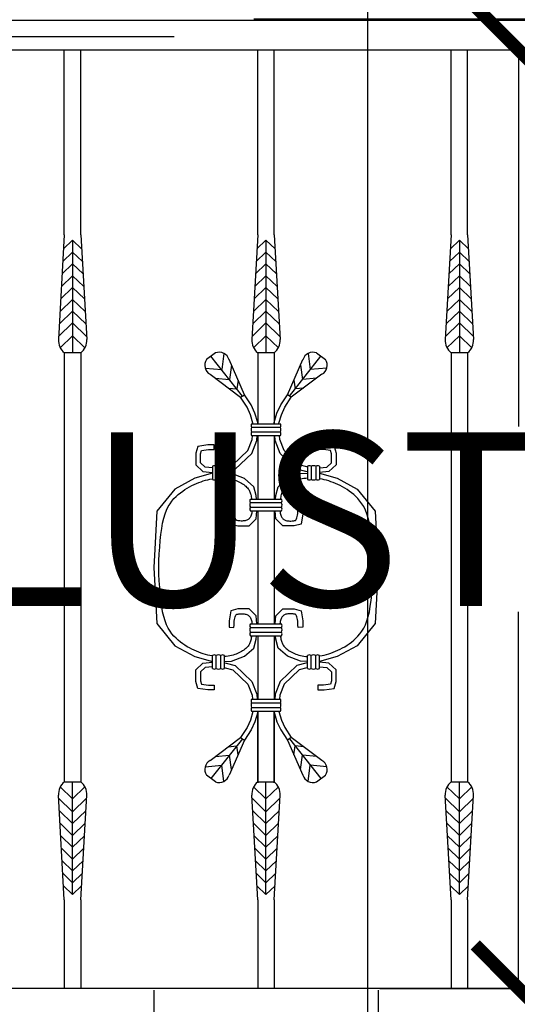
# Model space of a CAD drawing. Units: inches. Extents: x 2278 to 7495, y -71 to 1198.
# Tile 24 of 44: x 5084 to 5101, y 126 to 160. Entities that reach past the tile are written whole.
import ezdxf

# ---------------------------------------------------------------- set-up
doc = ezdxf.new("R2010")
doc.units = ezdxf.units.IN
doc.header["$MEASUREMENT"] = 0
doc.layers.add('A-ANNO-DIMS', color=2, linetype='Continuous', lineweight=18)
doc.layers.add('A-ELEV', color=7, linetype='Continuous', lineweight=25)
doc.styles.get("Standard").update_dxf_attribs({"font": 'arial.ttf'})
doc.dimstyles.get("Standard").update_dxf_attribs({"dimtxt": 6, "dimasz": 3, "dimexe": 0.18, "dimexo": 0.0625, "dimgap": 0.09, "dimtad": 0, "dimtih": 1, "dimtoh": 1, "dimdec": 0, "dimzin": 0, "dimdsep": 46, "dimlunit": 3, "dimtxsty": 'Standard', "dimblk": 'ARCHTICK', "dimcen": 0.09, "dimadec": 0, "dimazin": 0, "dimtfac": 1, "dimtdec": 0, "dimtofl": 0, "dimtmove": 0, "dimatfit": 3, "dimfxl": 1, "dimtolj": 1, "dimtzin": 0, "dimarcsym": 0})

# ---------------------------------------------------------------- blocks, each defined once
blk = doc.blocks.new('BALUSTER-ORNATE-A')
for p, q in [((3.585, 26.003), (3.585, 32.384)), ((4.155, 26.003), (4.155, 32.38)), ((3.585, 26.003), (3.383, 22.393)), ((4.155, 26.003), (4.357, 22.393)), ((3.558, 25.516), (3.87, 25.818)), ((3.87, 25.818), (3.87, 21.929)), ((4.182, 25.516), (3.87, 25.818)), ((3.533, 25.084), (3.87, 25.41)), ((4.207, 25.084), (3.87, 25.41)), ((3.509, 24.653), (3.87, 25.001)), ((4.231, 24.653), (3.87, 25.001)), ((3.485, 24.221), (3.87, 24.593)), ((4.255, 24.221), (3.87, 24.593)), ((3.461, 23.79), (3.87, 24.185)), ((4.279, 23.79), (3.87, 24.185)), ((3.437, 23.358), (3.87, 23.777)), ((4.303, 23.358), (3.87, 23.777)), ((3.413, 22.927), (3.87, 23.369)), ((4.327, 22.927), (3.87, 23.369)), ((3.388, 22.495), (3.87, 22.961)), ((4.352, 22.495), (3.87, 22.961)), ((3.442, 22.106), (3.87, 22.52)), ((4.299, 22.106), (3.87, 22.52)), ((2.128, 21.929), (1.813, 21.699)), ((3.063, 20.442), (1.97, 21.814)), ((2.412, 21.914), (2.339, 21.352)), ((3.585, 21.929), (3.585, 19.485)), ((4.155, 21.929), (3.585, 21.929)), ((4.155, 21.929), (4.155, 19.485)), ((4.677, 20.442), (5.77, 21.814)), ((5.328, 21.914), (5.401, 21.352)), ((5.612, 21.929), (5.927, 21.699)), ((1.774, 21.406), (2.339, 21.352)), ((3.131, 20.487), (2.594, 21.696)), ((2.678, 21.507), (2.613, 21.007)), ((4.609, 20.487), (5.146, 21.696)), ((5.062, 21.507), (5.127, 21.007)), ((5.966, 21.406), (5.401, 21.352)), ((1.936, 21.192), (2.995, 20.398)), ((5.804, 21.192), (4.745, 20.398)), ((2.111, 21.055), (2.613, 21.007)), ((2.907, 20.992), (2.868, 20.688)), ((4.833, 20.992), (4.872, 20.688)), ((5.629, 21.055), (5.127, 21.007)), ((2.562, 20.717), (2.868, 20.688)), ((2.995, 20.398), (3.131, 20.487)), ((3.217, 20.057), (2.995, 20.398)), ((3.36, 20.135), (3.131, 20.487)), ((4.38, 20.135), (4.609, 20.487)), ((4.523, 20.057), (4.745, 20.398)), ((4.745, 20.398), (4.609, 20.487)), ((5.178, 20.717), (4.872, 20.688)), ((3.337, 19.795), (3.217, 20.057)), ((3.49, 19.852), (3.36, 20.135)), ((4.25, 19.852), (4.38, 20.135)), ((4.403, 19.795), (4.523, 20.057)), ((3.421, 19.506), (3.337, 19.795)), ((3.585, 19.526), (3.49, 19.852)), ((4.155, 19.526), (4.25, 19.852)), ((4.319, 19.506), (4.403, 19.795)), ((3.37, 19.485), (4.37, 19.485)), ((3.42, 19.485), (3.421, 19.506)), ((3.583, 19.485), (3.585, 19.526)), ((4.157, 19.485), (4.155, 19.526)), ((4.32, 19.485), (4.319, 19.506)), ((3.37, 19.363), (4.37, 19.363)), ((3.37, 19.2), (4.37, 19.2)), ((3.37, 19.077), (4.37, 19.077)), ((3.396, 18.942), (3.402, 19.077)), ((3.558, 18.908), (3.565, 19.077)), ((3.585, 19.077), (3.585, 16.887)), ((4.155, 19.077), (4.155, 16.887)), ((4.182, 18.908), (4.175, 19.077)), ((4.344, 18.942), (4.338, 19.077)), ((1.513, 18.705), (1.449, 18.469)), ((1.866, 18.759), (1.513, 18.705)), ((2.084, 18.759), (1.866, 18.759)), ((2.084, 18.596), (2.084, 18.759)), ((3.247, 18.557), (3.396, 18.942)), ((3.385, 18.463), (3.558, 18.908)), ((4.355, 18.463), (4.182, 18.908)), ((4.493, 18.557), (4.344, 18.942)), ((5.656, 18.596), (5.656, 18.759)), ((5.656, 18.759), (5.874, 18.759)), ((5.874, 18.759), (6.227, 18.705)), ((6.227, 18.705), (6.291, 18.469)), ((1.449, 18.469), (1.449, 18.069)), ((1.612, 18.447), (1.642, 18.56)), ((1.612, 18.138), (1.612, 18.447)), ((1.642, 18.56), (1.879, 18.596)), ((1.879, 18.596), (2.084, 18.596)), ((2.719, 18.062), (3.247, 18.557)), ((2.801, 17.915), (3.385, 18.463)), ((4.939, 17.915), (4.355, 18.463)), ((5.021, 18.062), (4.493, 18.557)), ((5.861, 18.596), (5.656, 18.596)), ((6.098, 18.56), (5.861, 18.596)), ((6.128, 18.447), (6.098, 18.56)), ((6.128, 18.138), (6.128, 18.447)), ((6.291, 18.469), (6.291, 18.069)), ((1.449, 18.069), (1.694, 17.833)), ((1.767, 17.989), (1.612, 18.138)), ((2.026, 18.021), (2.026, 17.565)), ((2.148, 18.021), (2.148, 17.565)), ((2.311, 18.021), (2.311, 17.565)), ((2.434, 18.021), (2.434, 17.565)), ((2.462, 17.993), (2.719, 18.062)), ((5.278, 17.993), (5.021, 18.062)), ((5.306, 18.021), (5.306, 17.565)), ((5.429, 18.021), (5.429, 17.565)), ((5.592, 18.021), (5.592, 17.565)), ((5.714, 18.021), (5.714, 17.565)), ((5.973, 17.989), (6.128, 18.138)), ((6.291, 18.069), (6.046, 17.833)), ((2.026, 17.782), (1.412, 17.603)), ((1.694, 17.833), (2.026, 17.797)), ((2.026, 17.961), (1.767, 17.989)), ((2.434, 17.99), (2.462, 17.993)), ((2.434, 17.826), (2.492, 17.833)), ((2.683, 17.766), (2.434, 17.777)), ((2.492, 17.833), (2.801, 17.915)), ((3.128, 17.594), (2.683, 17.766)), ((4.612, 17.594), (5.057, 17.766)), ((5.248, 17.833), (4.939, 17.915)), ((5.057, 17.766), (5.306, 17.777)), ((5.306, 17.826), (5.248, 17.833)), ((5.306, 17.99), (5.278, 17.993)), ((5.714, 17.961), (5.973, 17.989)), ((6.046, 17.833), (5.714, 17.797)), ((5.714, 17.782), (6.328, 17.603)), ((1.412, 17.603), (0.722, 17.231)), ((1.23, 17.309), (1.309, 17.35)), ((1.309, 17.35), (1.389, 17.388)), ((1.389, 17.388), (1.469, 17.422)), ((1.469, 17.422), (1.549, 17.454)), ((1.549, 17.454), (1.627, 17.484)), ((1.627, 17.484), (1.705, 17.51)), ((1.705, 17.51), (1.782, 17.533)), ((1.782, 17.533), (1.858, 17.553)), ((1.858, 17.553), (1.933, 17.571)), ((1.933, 17.571), (2.007, 17.585)), ((2.007, 17.585), (2.026, 17.587)), ((2.434, 17.606), (2.499, 17.6)), ((2.499, 17.6), (2.563, 17.592)), ((2.563, 17.592), (2.624, 17.582)), ((2.624, 17.582), (2.683, 17.57)), ((2.683, 17.57), (2.739, 17.556)), ((2.739, 17.556), (2.792, 17.54)), ((2.792, 17.54), (2.843, 17.522)), ((2.843, 17.522), (2.891, 17.503)), ((2.891, 17.503), (2.937, 17.482)), ((2.937, 17.482), (2.981, 17.46)), ((2.981, 17.46), (3.024, 17.436)), ((3.024, 17.436), (3.064, 17.41)), ((3.064, 17.41), (3.102, 17.384)), ((3.102, 17.384), (3.138, 17.357)), ((3.446, 17.313), (3.128, 17.594)), ((3.138, 17.357), (3.171, 17.329)), ((3.171, 17.329), (3.201, 17.301)), ((4.294, 17.313), (4.612, 17.594)), ((4.569, 17.329), (4.539, 17.301)), ((4.602, 17.357), (4.569, 17.329)), ((4.638, 17.384), (4.602, 17.357)), ((4.676, 17.41), (4.638, 17.384)), ((4.716, 17.436), (4.676, 17.41)), ((4.759, 17.46), (4.716, 17.436)), ((4.803, 17.482), (4.759, 17.46)), ((4.849, 17.503), (4.803, 17.482)), ((4.897, 17.522), (4.849, 17.503)), ((4.948, 17.54), (4.897, 17.522)), ((5.001, 17.556), (4.948, 17.54)), ((5.057, 17.57), (5.001, 17.556)), ((5.116, 17.582), (5.057, 17.57)), ((5.177, 17.592), (5.116, 17.582)), ((5.241, 17.6), (5.177, 17.592)), ((5.306, 17.606), (5.241, 17.6)), ((5.733, 17.585), (5.714, 17.587)), ((5.807, 17.571), (5.733, 17.585)), ((5.882, 17.553), (5.807, 17.571)), ((5.958, 17.533), (5.882, 17.553)), ((6.035, 17.51), (5.958, 17.533)), ((6.113, 17.484), (6.035, 17.51)), ((6.191, 17.454), (6.113, 17.484)), ((6.271, 17.422), (6.191, 17.454)), ((6.351, 17.388), (6.271, 17.422)), ((6.328, 17.603), (7.018, 17.231)), ((6.431, 17.35), (6.351, 17.388)), ((6.51, 17.309), (6.431, 17.35)), ((0.722, 17.231), (0.096, 16.469)), ((0.764, 16.975), (0.839, 17.043)), ((0.839, 17.043), (0.916, 17.105)), ((0.916, 17.105), (0.993, 17.163)), ((0.993, 17.163), (1.071, 17.216)), ((1.071, 17.216), (1.15, 17.265)), ((1.15, 17.265), (1.23, 17.309)), ((3.201, 17.301), (3.228, 17.272)), ((3.228, 17.272), (3.252, 17.244)), ((3.252, 17.244), (3.272, 17.217)), ((3.272, 17.217), (3.288, 17.19)), ((3.288, 17.19), (3.303, 17.162)), ((3.303, 17.162), (3.316, 17.134)), ((3.316, 17.134), (3.327, 17.104)), ((3.327, 17.104), (3.337, 17.072)), ((3.337, 17.072), (3.346, 17.038)), ((3.346, 17.038), (3.354, 17.001)), ((3.354, 17.001), (3.361, 16.962)), ((3.528, 17.004), (3.446, 17.313)), ((3.542, 16.887), (3.528, 17.004)), ((4.198, 16.887), (4.212, 17.004)), ((4.212, 17.004), (4.294, 17.313)), ((4.386, 17.001), (4.379, 16.962)), ((4.394, 17.038), (4.386, 17.001)), ((4.403, 17.072), (4.394, 17.038)), ((4.413, 17.104), (4.403, 17.072)), ((4.424, 17.134), (4.413, 17.104)), ((4.437, 17.162), (4.424, 17.134)), ((4.452, 17.19), (4.437, 17.162)), ((4.468, 17.217), (4.452, 17.19)), ((4.489, 17.244), (4.468, 17.217)), ((4.512, 17.272), (4.489, 17.244)), ((4.539, 17.301), (4.512, 17.272)), ((6.59, 17.265), (6.51, 17.309)), ((6.669, 17.216), (6.59, 17.265)), ((6.747, 17.163), (6.669, 17.216)), ((6.824, 17.105), (6.747, 17.163)), ((6.901, 17.043), (6.824, 17.105)), ((6.976, 16.975), (6.901, 17.043)), ((7.018, 17.231), (7.644, 16.469)), ((0.495, 16.624), (0.557, 16.727)), ((0.557, 16.727), (0.623, 16.819)), ((0.623, 16.819), (0.692, 16.9)), ((0.692, 16.9), (0.764, 16.975)), ((3.329, 16.887), (4.411, 16.887)), ((3.329, 16.764), (4.411, 16.764)), ((3.361, 16.962), (3.368, 16.922)), ((3.368, 16.922), (3.374, 16.887)), ((4.372, 16.922), (4.366, 16.887)), ((4.379, 16.962), (4.372, 16.922)), ((7.048, 16.9), (6.976, 16.975)), ((7.117, 16.819), (7.048, 16.9)), ((7.183, 16.727), (7.117, 16.819)), ((7.245, 16.624), (7.183, 16.727)), ((0.096, 16.469), (0.025, 15.162)), ((0.34, 16.227), (0.386, 16.376)), ((0.386, 16.376), (0.438, 16.508)), ((0.438, 16.508), (0.495, 16.624)), ((2.764, 16.599), (2.602, 16.596)), ((2.602, 16.596), (2.602, 16.378)), ((2.602, 16.378), (2.656, 16.024)), ((2.766, 16.522), (2.764, 16.599)), ((2.769, 16.452), (2.766, 16.522)), ((2.775, 16.388), (2.769, 16.452)), ((2.783, 16.331), (2.775, 16.388)), ((2.792, 16.28), (2.783, 16.331)), ((3.329, 16.601), (4.411, 16.601)), ((3.329, 16.479), (4.411, 16.479)), ((3.357, 16.329), (3.346, 16.299)), ((3.368, 16.364), (3.357, 16.329)), ((3.376, 16.401), (3.368, 16.364)), ((3.383, 16.441), (3.376, 16.401)), ((3.388, 16.479), (3.383, 16.441)), ((3.528, 16.206), (3.557, 16.479)), ((3.585, 16.479), (3.585, 12.578)), ((4.155, 16.479), (4.155, 12.578)), ((4.212, 16.206), (4.183, 16.479)), ((4.352, 16.479), (4.357, 16.441)), ((4.357, 16.441), (4.364, 16.401)), ((4.364, 16.401), (4.372, 16.364)), ((4.372, 16.364), (4.383, 16.329)), ((4.383, 16.329), (4.394, 16.299)), ((4.948, 16.28), (4.957, 16.331)), ((4.957, 16.331), (4.965, 16.388)), ((4.965, 16.388), (4.971, 16.452)), ((4.971, 16.452), (4.974, 16.522)), ((4.974, 16.522), (4.976, 16.599)), ((4.976, 16.599), (5.138, 16.596)), ((5.138, 16.378), (5.084, 16.024)), ((5.138, 16.596), (5.138, 16.378)), ((7.302, 16.508), (7.245, 16.624)), ((7.354, 16.376), (7.302, 16.508)), ((7.4, 16.227), (7.354, 16.376)), ((7.644, 16.469), (7.715, 15.162)), ((0.267, 15.87), (0.3, 16.057)), ((0.3, 16.057), (0.34, 16.227)), ((2.656, 16.024), (2.892, 15.961)), ((2.803, 16.237), (2.792, 16.28)), ((2.815, 16.203), (2.803, 16.237)), ((2.825, 16.18), (2.815, 16.203)), ((2.834, 16.166), (2.825, 16.18)), ((2.84, 16.159), (2.834, 16.166)), ((2.846, 16.154), (2.84, 16.159)), ((2.852, 16.151), (2.846, 16.154)), ((2.863, 16.146), (2.852, 16.151)), ((2.88, 16.142), (2.863, 16.146)), ((2.905, 16.137), (2.88, 16.142)), ((2.936, 16.134), (2.905, 16.137)), ((2.971, 16.131), (2.936, 16.134)), ((3.008, 16.129), (2.971, 16.131)), ((3.045, 16.129), (3.008, 16.129)), ((3.081, 16.13), (3.045, 16.129)), ((3.117, 16.133), (3.081, 16.13)), ((3.15, 16.138), (3.117, 16.133)), ((3.179, 16.145), (3.15, 16.138)), ((3.205, 16.154), (3.179, 16.145)), ((3.228, 16.164), (3.205, 16.154)), ((3.249, 16.176), (3.228, 16.164)), ((3.268, 16.19), (3.249, 16.176)), ((3.286, 16.207), (3.268, 16.19)), ((3.303, 16.225), (3.286, 16.207)), ((3.292, 15.961), (3.528, 16.206)), ((3.318, 16.247), (3.303, 16.225)), ((3.333, 16.271), (3.318, 16.247)), ((3.346, 16.299), (3.333, 16.271)), ((4.448, 15.961), (4.212, 16.206)), ((4.394, 16.299), (4.407, 16.271)), ((4.407, 16.271), (4.422, 16.247)), ((4.422, 16.247), (4.437, 16.225)), ((4.437, 16.225), (4.454, 16.207)), ((4.454, 16.207), (4.472, 16.19)), ((4.472, 16.19), (4.491, 16.176)), ((4.491, 16.176), (4.512, 16.164)), ((4.512, 16.164), (4.535, 16.154)), ((4.535, 16.154), (4.561, 16.145)), ((4.561, 16.145), (4.59, 16.138)), ((4.59, 16.138), (4.623, 16.133)), ((4.623, 16.133), (4.659, 16.13)), ((4.659, 16.13), (4.695, 16.129)), ((4.695, 16.129), (4.732, 16.129)), ((4.732, 16.129), (4.769, 16.131)), ((4.769, 16.131), (4.804, 16.134)), ((4.804, 16.134), (4.835, 16.137)), ((4.835, 16.137), (4.86, 16.142)), ((5.084, 16.024), (4.848, 15.961)), ((4.86, 16.142), (4.877, 16.146)), ((4.877, 16.146), (4.888, 16.151)), ((4.888, 16.151), (4.895, 16.154)), ((4.895, 16.154), (4.9, 16.159)), ((4.9, 16.159), (4.906, 16.166)), ((4.906, 16.166), (4.915, 16.18)), ((4.915, 16.18), (4.925, 16.203)), ((4.925, 16.203), (4.937, 16.237)), ((4.937, 16.237), (4.948, 16.28)), ((7.44, 16.057), (7.4, 16.227)), ((7.473, 15.87), (7.44, 16.057)), ((0.217, 15.452), (0.239, 15.667)), ((0.239, 15.667), (0.267, 15.87)), ((2.892, 15.961), (3.292, 15.961)), ((4.848, 15.961), (4.448, 15.961)), ((7.501, 15.667), (7.473, 15.87)), ((7.523, 15.452), (7.501, 15.667)), ((0.199, 15.227), (0.217, 15.452)), ((7.541, 15.227), (7.523, 15.452)), ((0.025, 15.162), (0, 14.529)), ((0.173, 14.759), (0.185, 14.995)), ((0.185, 14.995), (0.199, 15.227)), ((7.555, 14.995), (7.541, 15.227)), ((7.567, 14.759), (7.555, 14.995)), ((7.715, 15.162), (7.74, 14.529)), ((0.163, 14.522), (0.173, 14.759)), ((7.577, 14.522), (7.567, 14.759)), ((0, 14.529), (0.025, 13.895)), ((0.173, 14.298), (0.163, 14.536)), ((0.185, 14.062), (0.173, 14.298)), ((7.555, 14.062), (7.567, 14.298)), ((7.567, 14.298), (7.577, 14.536)), ((7.74, 14.529), (7.715, 13.895)), ((0.199, 13.831), (0.185, 14.062)), ((7.541, 13.831), (7.555, 14.062)), ((0.025, 13.895), (0.096, 12.589)), ((0.217, 13.606), (0.199, 13.831)), ((0.239, 13.391), (0.217, 13.606)), ((7.501, 13.391), (7.523, 13.606)), ((7.523, 13.606), (7.541, 13.831)), ((7.715, 13.895), (7.644, 12.589)), ((0.267, 13.188), (0.239, 13.391)), ((7.473, 13.188), (7.501, 13.391)), ((0.3, 13), (0.267, 13.188)), ((0.34, 12.831), (0.3, 13)), ((2.656, 13.033), (2.602, 12.679)), ((2.892, 13.097), (2.656, 13.033)), ((2.852, 12.907), (2.863, 12.911)), ((2.863, 12.911), (2.88, 12.916)), ((2.88, 12.916), (2.905, 12.92)), ((3.292, 13.097), (2.892, 13.097)), ((2.905, 12.92), (2.936, 12.924)), ((2.936, 12.924), (2.971, 12.927)), ((2.971, 12.927), (3.008, 12.929)), ((3.008, 12.929), (3.045, 12.929)), ((3.045, 12.929), (3.081, 12.928)), ((3.081, 12.928), (3.117, 12.924)), ((3.117, 12.924), (3.15, 12.919)), ((3.15, 12.919), (3.179, 12.912)), ((3.179, 12.912), (3.205, 12.904)), ((3.528, 12.852), (3.292, 13.097)), ((4.212, 12.852), (4.448, 13.097)), ((4.448, 13.097), (4.848, 13.097)), ((4.561, 12.912), (4.535, 12.904)), ((4.59, 12.919), (4.561, 12.912)), ((4.623, 12.924), (4.59, 12.919)), ((4.659, 12.928), (4.623, 12.924)), ((4.695, 12.929), (4.659, 12.928)), ((4.732, 12.929), (4.695, 12.929)), ((4.769, 12.927), (4.732, 12.929)), ((4.804, 12.924), (4.769, 12.927)), ((4.835, 12.92), (4.804, 12.924)), ((4.86, 12.916), (4.835, 12.92)), ((4.848, 13.097), (5.084, 13.033)), ((4.877, 12.911), (4.86, 12.916)), ((4.888, 12.907), (4.877, 12.911)), ((5.084, 13.033), (5.138, 12.679)), ((7.4, 12.831), (7.44, 13)), ((7.44, 13), (7.473, 13.188)), ((0.096, 12.589), (0.722, 11.827)), ((0.386, 12.681), (0.34, 12.831)), ((0.438, 12.549), (0.386, 12.681)), ((2.602, 12.679), (2.602, 12.462)), ((2.766, 12.536), (2.769, 12.605)), ((2.769, 12.605), (2.775, 12.669)), ((2.775, 12.669), (2.783, 12.727)), ((2.783, 12.727), (2.792, 12.778)), ((2.792, 12.778), (2.803, 12.82)), ((2.803, 12.82), (2.815, 12.854)), ((2.815, 12.854), (2.825, 12.878)), ((2.825, 12.878), (2.834, 12.892)), ((2.834, 12.892), (2.84, 12.899)), ((2.84, 12.899), (2.846, 12.903)), ((2.846, 12.903), (2.852, 12.907)), ((3.205, 12.904), (3.228, 12.893)), ((3.228, 12.893), (3.249, 12.881)), ((3.249, 12.881), (3.268, 12.867)), ((3.268, 12.867), (3.286, 12.851)), ((3.286, 12.851), (3.303, 12.832)), ((3.303, 12.832), (3.318, 12.811)), ((3.318, 12.811), (3.333, 12.786)), ((3.329, 12.578), (4.411, 12.578)), ((3.333, 12.786), (3.346, 12.759)), ((3.346, 12.759), (3.357, 12.728)), ((3.357, 12.728), (3.368, 12.694)), ((3.368, 12.694), (3.376, 12.656)), ((3.376, 12.656), (3.383, 12.616)), ((3.383, 12.616), (3.388, 12.578)), ((3.557, 12.578), (3.528, 12.852)), ((4.183, 12.578), (4.212, 12.852)), ((4.357, 12.616), (4.352, 12.578)), ((4.364, 12.656), (4.357, 12.616)), ((4.372, 12.694), (4.364, 12.656)), ((4.383, 12.728), (4.372, 12.694)), ((4.394, 12.759), (4.383, 12.728)), ((4.407, 12.786), (4.394, 12.759)), ((4.422, 12.811), (4.407, 12.786)), ((4.437, 12.832), (4.422, 12.811)), ((4.454, 12.851), (4.437, 12.832)), ((4.472, 12.867), (4.454, 12.851)), ((4.491, 12.881), (4.472, 12.867)), ((4.512, 12.893), (4.491, 12.881)), ((4.535, 12.904), (4.512, 12.893)), ((4.895, 12.903), (4.888, 12.907)), ((4.9, 12.899), (4.895, 12.903)), ((4.906, 12.892), (4.9, 12.899)), ((4.915, 12.878), (4.906, 12.892)), ((4.925, 12.854), (4.915, 12.878)), ((4.937, 12.82), (4.925, 12.854)), ((4.948, 12.778), (4.937, 12.82)), ((4.957, 12.727), (4.948, 12.778)), ((4.965, 12.669), (4.957, 12.727)), ((4.971, 12.605), (4.965, 12.669)), ((4.974, 12.536), (4.971, 12.605)), ((5.138, 12.679), (5.138, 12.462)), ((7.644, 12.589), (7.018, 11.827)), ((7.302, 12.549), (7.354, 12.681)), ((7.354, 12.681), (7.4, 12.831)), ((0.495, 12.433), (0.438, 12.549)), ((0.557, 12.33), (0.495, 12.433)), ((0.623, 12.239), (0.557, 12.33)), ((0.692, 12.157), (0.623, 12.239)), ((2.602, 12.462), (2.764, 12.459)), ((2.764, 12.459), (2.766, 12.536)), ((3.329, 12.456), (4.411, 12.456)), ((3.329, 12.293), (4.411, 12.293)), ((4.976, 12.459), (4.974, 12.536)), ((5.138, 12.462), (4.976, 12.459)), ((7.048, 12.157), (7.117, 12.239)), ((7.117, 12.239), (7.183, 12.33)), ((7.183, 12.33), (7.245, 12.433)), ((7.245, 12.433), (7.302, 12.549)), ((0.764, 12.083), (0.692, 12.157)), ((0.839, 12.015), (0.764, 12.083)), ((0.916, 11.952), (0.839, 12.015)), ((0.993, 11.894), (0.916, 11.952)), ((1.071, 11.841), (0.993, 11.894)), ((3.303, 11.895), (3.288, 11.868)), ((3.316, 11.924), (3.303, 11.895)), ((3.327, 11.954), (3.316, 11.924)), ((3.337, 11.986), (3.327, 11.954)), ((3.329, 12.171), (4.411, 12.171)), ((3.346, 12.02), (3.337, 11.986)), ((3.354, 12.056), (3.346, 12.02)), ((3.361, 12.095), (3.354, 12.056)), ((3.368, 12.136), (3.361, 12.095)), ((3.374, 12.171), (3.368, 12.136)), ((3.446, 11.745), (3.528, 12.053)), ((3.528, 12.053), (3.542, 12.171)), ((3.585, 12.171), (3.585, 9.98)), ((4.155, 12.171), (4.155, 9.98)), ((4.212, 12.053), (4.198, 12.171)), ((4.294, 11.745), (4.212, 12.053)), ((4.366, 12.171), (4.372, 12.136)), ((4.372, 12.136), (4.379, 12.095)), ((4.379, 12.095), (4.386, 12.056)), ((4.386, 12.056), (4.394, 12.02)), ((4.394, 12.02), (4.403, 11.986)), ((4.403, 11.986), (4.413, 11.954)), ((4.413, 11.954), (4.424, 11.924)), ((4.424, 11.924), (4.437, 11.895)), ((4.437, 11.895), (4.452, 11.868)), ((6.669, 11.841), (6.747, 11.894)), ((6.747, 11.894), (6.824, 11.952)), ((6.824, 11.952), (6.901, 12.015)), ((6.901, 12.015), (6.976, 12.083)), ((6.976, 12.083), (7.048, 12.157)), ((0.722, 11.827), (1.412, 11.455)), ((1.15, 11.793), (1.071, 11.841)), ((1.23, 11.748), (1.15, 11.793)), ((1.309, 11.708), (1.23, 11.748)), ((1.389, 11.67), (1.309, 11.708)), ((1.469, 11.635), (1.389, 11.67)), ((1.549, 11.603), (1.469, 11.635)), ((1.627, 11.574), (1.549, 11.603)), ((1.705, 11.548), (1.627, 11.574)), ((2.891, 11.555), (2.843, 11.535)), ((2.937, 11.576), (2.891, 11.555)), ((2.981, 11.598), (2.937, 11.576)), ((3.024, 11.622), (2.981, 11.598)), ((3.064, 11.647), (3.024, 11.622)), ((3.102, 11.673), (3.064, 11.647)), ((3.138, 11.701), (3.102, 11.673)), ((3.128, 11.464), (3.446, 11.745)), ((3.171, 11.729), (3.138, 11.701)), ((3.201, 11.757), (3.171, 11.729)), ((3.228, 11.785), (3.201, 11.757)), ((3.252, 11.813), (3.228, 11.785)), ((3.272, 11.841), (3.252, 11.813)), ((3.288, 11.868), (3.272, 11.841)), ((4.612, 11.464), (4.294, 11.745)), ((4.452, 11.868), (4.468, 11.841)), ((4.468, 11.841), (4.489, 11.813)), ((4.489, 11.813), (4.512, 11.785)), ((4.512, 11.785), (4.539, 11.757)), ((4.539, 11.757), (4.569, 11.729)), ((4.569, 11.729), (4.602, 11.701)), ((4.602, 11.701), (4.638, 11.673)), ((4.638, 11.673), (4.676, 11.647)), ((4.676, 11.647), (4.716, 11.622)), ((4.716, 11.622), (4.759, 11.598)), ((4.759, 11.598), (4.803, 11.576)), ((4.803, 11.576), (4.849, 11.555)), ((4.849, 11.555), (4.897, 11.535)), ((6.035, 11.548), (6.113, 11.574)), ((6.113, 11.574), (6.191, 11.603)), ((6.191, 11.603), (6.271, 11.635)), ((6.271, 11.635), (6.351, 11.67)), ((7.018, 11.827), (6.328, 11.455)), ((6.351, 11.67), (6.431, 11.708)), ((6.431, 11.708), (6.51, 11.748)), ((6.51, 11.748), (6.59, 11.793)), ((6.59, 11.793), (6.669, 11.841)), ((1.412, 11.455), (2.026, 11.276)), ((1.449, 10.988), (1.694, 11.225)), ((1.694, 11.225), (2.026, 11.261)), ((1.782, 11.524), (1.705, 11.548)), ((1.858, 11.504), (1.782, 11.524)), ((1.933, 11.487), (1.858, 11.504)), ((2.007, 11.473), (1.933, 11.487)), ((2.026, 11.47), (2.007, 11.473)), ((2.026, 11.037), (2.026, 11.493)), ((2.148, 11.037), (2.148, 11.493)), ((2.311, 11.037), (2.311, 11.493)), ((2.434, 11.037), (2.434, 11.493)), ((2.499, 11.457), (2.434, 11.451)), ((2.434, 11.28), (2.683, 11.291)), ((2.434, 11.232), (2.492, 11.225)), ((2.492, 11.225), (2.801, 11.143)), ((2.563, 11.465), (2.499, 11.457)), ((2.624, 11.476), (2.563, 11.465)), ((2.683, 11.488), (2.624, 11.476)), ((2.739, 11.502), (2.683, 11.488)), ((2.683, 11.291), (3.128, 11.464)), ((2.792, 11.518), (2.739, 11.502)), ((2.843, 11.535), (2.792, 11.518)), ((5.057, 11.291), (4.612, 11.464)), ((4.897, 11.535), (4.948, 11.518)), ((5.248, 11.225), (4.939, 11.143)), ((4.948, 11.518), (5.001, 11.502)), ((5.001, 11.502), (5.057, 11.488)), ((5.057, 11.488), (5.116, 11.476)), ((5.306, 11.28), (5.057, 11.291)), ((5.116, 11.476), (5.177, 11.465)), ((5.177, 11.465), (5.241, 11.457)), ((5.241, 11.457), (5.306, 11.451)), ((5.306, 11.232), (5.248, 11.225)), ((5.306, 11.037), (5.306, 11.493)), ((5.429, 11.037), (5.429, 11.493)), ((5.592, 11.037), (5.592, 11.493)), ((5.714, 11.037), (5.714, 11.493)), ((5.714, 11.47), (5.733, 11.473)), ((6.328, 11.455), (5.714, 11.276)), ((6.046, 11.225), (5.714, 11.261)), ((5.733, 11.473), (5.807, 11.487)), ((5.807, 11.487), (5.882, 11.504)), ((5.882, 11.504), (5.958, 11.524)), ((5.958, 11.524), (6.035, 11.548)), ((6.291, 10.988), (6.046, 11.225)), ((1.449, 10.589), (1.449, 10.988)), ((1.767, 11.069), (1.612, 10.919)), ((1.612, 10.919), (1.612, 10.611)), ((2.026, 11.097), (1.767, 11.069)), ((2.434, 11.067), (2.462, 11.064)), ((2.462, 11.064), (2.719, 10.996)), ((2.719, 10.996), (3.247, 10.501)), ((2.801, 11.143), (3.385, 10.594)), ((4.939, 11.143), (4.355, 10.594)), ((5.021, 10.996), (4.493, 10.501)), ((5.278, 11.064), (5.021, 10.996)), ((5.306, 11.067), (5.278, 11.064)), ((5.714, 11.097), (5.973, 11.069)), ((5.973, 11.069), (6.128, 10.919)), ((6.128, 10.919), (6.128, 10.611)), ((6.291, 10.589), (6.291, 10.988)), ((1.513, 10.353), (1.449, 10.589)), ((1.612, 10.611), (1.642, 10.498)), ((3.385, 10.594), (3.558, 10.149)), ((4.355, 10.594), (4.182, 10.149)), ((6.128, 10.611), (6.098, 10.498)), ((6.227, 10.353), (6.291, 10.589)), ((1.866, 10.298), (1.513, 10.353)), ((1.642, 10.498), (1.879, 10.461)), ((2.084, 10.298), (1.866, 10.298)), ((1.879, 10.461), (2.084, 10.461)), ((2.084, 10.461), (2.084, 10.298)), ((3.247, 10.501), (3.396, 10.115)), ((4.493, 10.501), (4.344, 10.115)), ((5.861, 10.461), (5.656, 10.461)), ((5.656, 10.461), (5.656, 10.298)), ((5.656, 10.298), (5.874, 10.298)), ((6.098, 10.498), (5.861, 10.461)), ((5.874, 10.298), (6.227, 10.353)), ((3.37, 9.98), (4.37, 9.98)), ((3.37, 9.858), (4.37, 9.858)), ((3.396, 10.115), (3.402, 9.98)), ((3.558, 10.149), (3.565, 9.98)), ((4.182, 10.149), (4.175, 9.98)), ((4.344, 10.115), (4.338, 9.98)), ((3.421, 9.552), (3.337, 9.262)), ((3.37, 9.695), (4.37, 9.695)), ((3.37, 9.573), (4.37, 9.573)), ((3.42, 9.573), (3.421, 9.552)), ((3.585, 9.532), (3.49, 9.205)), ((3.583, 9.573), (3.585, 9.532)), ((3.585, 9.573), (3.585, 7.095)), ((3.585, 7.095), (3.585, 9.573)), ((4.155, 9.573), (4.155, 7.095)), ((4.155, 7.095), (4.155, 9.573)), ((4.157, 9.573), (4.155, 9.532)), ((4.155, 9.532), (4.25, 9.205)), ((4.32, 9.573), (4.319, 9.552)), ((4.319, 9.552), (4.403, 9.262)), ((3.337, 9.262), (3.217, 9.001)), ((3.49, 9.205), (3.36, 8.922)), ((4.25, 9.205), (4.38, 8.922)), ((4.403, 9.262), (4.523, 9.001)), ((3.217, 9.001), (2.995, 8.66)), ((3.36, 8.922), (3.131, 8.571)), ((4.38, 8.922), (4.609, 8.571)), ((4.523, 9.001), (4.745, 8.66)), ((1.936, 7.866), (2.995, 8.66)), ((3.063, 8.615), (1.97, 7.244)), ((3.131, 8.571), (2.594, 7.362)), ((2.995, 8.66), (3.131, 8.571)), ((4.745, 8.66), (4.609, 8.571)), ((4.609, 8.571), (5.146, 7.362)), ((4.677, 8.615), (5.77, 7.244)), ((5.804, 7.866), (4.745, 8.66)), ((2.562, 8.34), (2.868, 8.37)), ((2.907, 8.066), (2.868, 8.37)), ((4.833, 8.066), (4.872, 8.37)), ((5.178, 8.34), (4.872, 8.37)), ((2.111, 8.002), (2.613, 8.051)), ((2.678, 7.551), (2.613, 8.051)), ((5.062, 7.551), (5.127, 8.051)), ((5.629, 8.002), (5.127, 8.051)), ((1.774, 7.651), (2.339, 7.706)), ((2.412, 7.143), (2.339, 7.706)), ((5.328, 7.143), (5.401, 7.706)), ((5.966, 7.651), (5.401, 7.706)), ((2.128, 7.128), (1.813, 7.359)), ((5.612, 7.128), (5.927, 7.359)), ((3.442, 6.952), (3.87, 6.538)), ((3.585, 7.128), (4.155, 7.128)), ((3.87, 3.24), (3.87, 7.128)), ((4.299, 6.952), (3.87, 6.538)), ((3.585, 3.055), (3.383, 6.664)), ((3.388, 6.562), (3.87, 6.097)), ((4.352, 6.562), (3.87, 6.097)), ((4.155, 3.055), (4.357, 6.664)), ((3.413, 6.131), (3.87, 5.689)), ((4.327, 6.131), (3.87, 5.689)), ((3.437, 5.699), (3.87, 5.28)), ((4.303, 5.699), (3.87, 5.28)), ((3.461, 5.268), (3.87, 4.872)), ((4.279, 5.268), (3.87, 4.872)), ((3.485, 4.836), (3.87, 4.464)), ((4.255, 4.836), (3.87, 4.464)), ((3.509, 4.405), (3.87, 4.056)), ((4.231, 4.405), (3.87, 4.056)), ((3.533, 3.973), (3.87, 3.648)), ((4.207, 3.973), (3.87, 3.648)), ((3.558, 3.542), (3.87, 3.24)), ((4.182, 3.542), (3.87, 3.24)), ((3.585, 3.055), (3.585, 0)), ((4.155, 3.055), (4.155, 0))]:
    blk.add_line(p, q)
for centre, radius, start, end in [((3.929, 22.355), 0.547, 176.0178, 231.0717), ((3.811, 22.355), 0.547, 308.9283, 3.9822), ((2.253, 21.595), 0.356, 16.4025, 110.5063), ((5.487, 21.595), 0.356, 69.4937, 163.5975), ((2.111, 21.502), 0.356, 146.575, 240.6788), ((5.629, 21.502), 0.356, 299.3212, 33.425), ((3.475, 19.424), 0.121, 149.7768, 210.2232), ((4.265, 19.424), 0.121, 329.7768, 30.2232), ((3.563, 19.281), 0.209, 157.1017, 202.8983), ((3.475, 19.139), 0.121, 149.7768, 210.2232), ((4.177, 19.281), 0.209, 337.1017, 22.8983), ((4.265, 19.139), 0.121, 329.7768, 30.2232), ((2.087, 17.916), 0.121, 59.7768, 120.2232), ((2.23, 17.828), 0.209, 67.1017, 112.8983), ((2.373, 17.916), 0.121, 59.7768, 120.2232), ((5.368, 17.916), 0.121, 59.7768, 120.2232), ((5.51, 17.828), 0.209, 67.1017, 112.8983), ((5.653, 17.916), 0.121, 59.7768, 120.2232), ((2.087, 17.67), 0.121, 239.7768, 300.2232), ((2.23, 17.758), 0.209, 247.1017, 292.8983), ((2.373, 17.67), 0.121, 239.7768, 300.2232), ((5.368, 17.67), 0.121, 239.7768, 300.2232), ((5.51, 17.758), 0.209, 247.1017, 292.8983), ((5.653, 17.67), 0.121, 239.7768, 300.2232), ((3.434, 16.825), 0.121, 149.7768, 210.2232), ((3.522, 16.683), 0.209, 157.1017, 202.8983), ((4.306, 16.825), 0.121, 329.7768, 30.2232), ((4.218, 16.683), 0.209, 337.1017, 22.8983), ((3.434, 16.54), 0.121, 149.7768, 210.2232), ((4.306, 16.54), 0.121, 329.7768, 30.2232), ((3.434, 12.517), 0.121, 149.7768, 210.2232), ((4.306, 12.517), 0.121, 329.7768, 30.2232), ((3.522, 12.375), 0.209, 157.1017, 202.8983), ((3.434, 12.232), 0.121, 149.7768, 210.2232), ((4.218, 12.375), 0.209, 337.1017, 22.8983), ((4.306, 12.232), 0.121, 329.7768, 30.2232), ((2.087, 11.388), 0.121, 59.7768, 120.2232), ((2.23, 11.3), 0.209, 67.1017, 112.8983), ((2.373, 11.388), 0.121, 59.7768, 120.2232), ((5.368, 11.388), 0.121, 59.7768, 120.2232), ((5.51, 11.3), 0.209, 67.1017, 112.8983), ((5.653, 11.388), 0.121, 59.7768, 120.2232), ((2.087, 11.142), 0.121, 239.7768, 300.2232), ((2.23, 11.23), 0.209, 247.1017, 292.8983), ((2.373, 11.142), 0.121, 239.7768, 300.2232), ((5.368, 11.142), 0.121, 239.7768, 300.2232), ((5.51, 11.23), 0.209, 247.1017, 292.8983), ((5.653, 11.142), 0.121, 239.7768, 300.2232), ((3.475, 9.919), 0.121, 149.7768, 210.2232), ((3.563, 9.776), 0.209, 157.1017, 202.8983), ((4.265, 9.919), 0.121, 329.7768, 30.2232), ((4.177, 9.776), 0.209, 337.1017, 22.8983), ((3.475, 9.634), 0.121, 149.7768, 210.2232), ((4.265, 9.634), 0.121, 329.7768, 30.2232), ((2.111, 7.555), 0.356, 119.3212, 213.425), ((5.629, 7.555), 0.356, 326.575, 60.6788), ((2.253, 7.462), 0.356, 249.4937, 343.5975), ((5.487, 7.462), 0.356, 196.4025, 290.5063), ((3.929, 6.703), 0.547, 128.9283, 183.9822), ((3.811, 6.703), 0.547, 356.0178, 51.0717)]:
    blk.add_arc(centre, radius, start, end)
blk = doc.blocks.new('RAIL-BAR-A')
for p, q in [((0.202, 26.003), (0.202, 32.38)), ((0.773, 26.003), (0.773, 32.38)), ((0.202, 26.003), (0, 22.393)), ((0.773, 26.003), (0.975, 22.393)), ((0.175, 25.516), (0.488, 25.818)), ((0.488, 25.818), (0.488, 21.929)), ((0.8, 25.516), (0.488, 25.818)), ((0.151, 25.084), (0.488, 25.41)), ((0.824, 25.084), (0.488, 25.41)), ((0.127, 24.653), (0.488, 25.001)), ((0.848, 24.653), (0.488, 25.001)), ((0.103, 24.221), (0.488, 24.593)), ((0.873, 24.221), (0.488, 24.593)), ((0.079, 23.79), (0.488, 24.185)), ((0.897, 23.79), (0.488, 24.185)), ((0.054, 23.358), (0.488, 23.777)), ((0.921, 23.358), (0.488, 23.777)), ((0.03, 22.927), (0.488, 23.369)), ((0.945, 22.927), (0.488, 23.369)), ((0.006, 22.495), (0.488, 22.961)), ((0.969, 22.495), (0.488, 22.961)), ((0.059, 22.106), (0.488, 22.52)), ((0.916, 22.106), (0.488, 22.52)), ((0.202, 21.929), (0.202, 7.128)), ((0.773, 21.929), (0.202, 21.929)), ((0.773, 21.929), (0.773, 7.128)), ((0.059, 6.952), (0.488, 6.538)), ((0.202, 7.128), (0.773, 7.128)), ((0.488, 3.24), (0.488, 7.128)), ((0.916, 6.952), (0.488, 6.538)), ((0.202, 3.055), (0, 6.664)), ((0.006, 6.562), (0.488, 6.097)), ((0.969, 6.562), (0.488, 6.097)), ((0.773, 3.055), (0.975, 6.664)), ((0.03, 6.131), (0.488, 5.689)), ((0.945, 6.131), (0.488, 5.689)), ((0.054, 5.699), (0.488, 5.28)), ((0.921, 5.699), (0.488, 5.28)), ((0.079, 5.268), (0.488, 4.872)), ((0.897, 5.268), (0.488, 4.872)), ((0.103, 4.836), (0.488, 4.464)), ((0.873, 4.836), (0.488, 4.464)), ((0.127, 4.405), (0.488, 4.056)), ((0.848, 4.405), (0.488, 4.056)), ((0.151, 3.973), (0.488, 3.648)), ((0.824, 3.973), (0.488, 3.648)), ((0.175, 3.542), (0.488, 3.24)), ((0.8, 3.542), (0.488, 3.24)), ((0.202, 3.055), (0.202, 0)), ((0.773, 3.055), (0.773, 0))]:
    blk.add_line(p, q)
for centre, start, end in [((0.546, 22.355), 176.0178, 231.0717), ((0.429, 22.355), 308.9283, 3.9822), ((0.546, 6.703), 128.9283, 183.9822), ((0.429, 6.703), 356.0178, 51.0717)]:
    blk.add_arc(centre, 0.547, start, end)
blk = doc.blocks.new('RAIL-BAR-B')
for p, q in [((17.353, 32.832), (1.059, 32.832)), ((0.203, 26.003), (0.203, 32.38)), ((0.773, 26.003), (0.773, 32.38)), ((0.203, 26.003), (0.001, 22.393)), ((0.773, 26.003), (0.976, 22.393)), ((0.176, 25.516), (0.488, 25.818)), ((0.488, 25.818), (0.488, 21.929)), ((0.801, 25.516), (0.488, 25.818)), ((0.152, 25.084), (0.488, 25.41)), ((0.825, 25.084), (0.488, 25.41)), ((0.128, 24.653), (0.488, 25.001)), ((0.849, 24.653), (0.488, 25.001)), ((0.103, 24.221), (0.488, 24.593)), ((0.873, 24.221), (0.488, 24.593)), ((0.079, 23.79), (0.488, 24.185)), ((0.897, 23.79), (0.488, 24.185)), ((0.055, 23.358), (0.488, 23.777)), ((0.922, 23.358), (0.488, 23.777)), ((0.031, 22.927), (0.488, 23.369)), ((0.946, 22.927), (0.488, 23.369)), ((0.007, 22.495), (0.488, 22.961)), ((0.97, 22.495), (0.488, 22.961)), ((0.06, 22.106), (0.488, 22.52)), ((0.917, 22.106), (0.488, 22.52)), ((0.203, 21.929), (0.203, 7.128)), ((0.773, 21.929), (0.203, 21.929)), ((0.773, 21.929), (0.773, 7.128)), ((0.06, 6.952), (0.488, 6.538)), ((0.203, 7.128), (0.773, 7.128)), ((0.488, 3.24), (0.488, 7.128)), ((0.917, 6.952), (0.488, 6.538)), ((0.203, 3.055), (0.001, 6.664)), ((0.007, 6.562), (0.488, 6.097)), ((0.97, 6.562), (0.488, 6.097)), ((0.773, 3.055), (0.976, 6.664)), ((0.031, 6.131), (0.488, 5.689)), ((0.946, 6.131), (0.488, 5.689)), ((0.055, 5.699), (0.488, 5.28)), ((0.922, 5.699), (0.488, 5.28)), ((0.079, 5.268), (0.488, 4.872)), ((0.897, 5.268), (0.488, 4.872)), ((0.103, 4.836), (0.488, 4.464)), ((0.873, 4.836), (0.488, 4.464)), ((0.128, 4.405), (0.488, 4.056)), ((0.849, 4.405), (0.488, 4.056)), ((0.152, 3.973), (0.488, 3.648)), ((0.825, 3.973), (0.488, 3.648)), ((0.176, 3.542), (0.488, 3.24)), ((0.801, 3.542), (0.488, 3.24)), ((0.203, 3.055), (0.203, 0)), ((0.773, 3.055), (0.773, 0))]:
    blk.add_line(p, q)
for centre, start, end in [((0.547, 22.355), 176.0178, 231.0717), ((0.429, 22.355), 308.9283, 3.9822), ((0.547, 6.703), 128.9283, 183.9822), ((0.429, 6.703), 356.0178, 51.0717)]:
    blk.add_arc(centre, 0.547, start, end)
blk = doc.blocks.new('_ArchTick')
at = {"color": 0, "linetype": 'ByBlock', "const_width": 0.15}
blk.add_lwpolyline([(-0.5, -0.5), (0.5, 0.5)], dxfattribs=at)
blk = doc.blocks.new('*D59')
at = {"layer": 'A-ANNO-DIMS', "color": 0, "lineweight": -2, "transparency": 16777216}
for p, q in [((5096.589, 159.183), (5101.564, 159.183)), ((5101.384, 159.183), (5101.384, 146.185)), ((5101.384, 126.799), (5101.384, 139.796)), ((5096.589, 126.799), (5101.564, 126.799))]:
    blk.add_line(p, q, dxfattribs=at)
at = {"layer": 'Defpoints', "color": 0, "transparency": 16777216}
for p in [(5096.527, 159.183), (5101.384, 159.183), (5096.527, 126.799)]:
    blk.add_point(p, dxfattribs=at)
at = {"layer": 'A-ANNO-DIMS', "color": 0, "lineweight": -2, "transparency": 16777216, "xscale": 3, "yscale": 3, "zscale": 3}
for p, rotation in [((5101.384, 159.183), 90), ((5101.384, 126.799), 270)]:
    blk.add_blockref('_ArchTick', p, dxfattribs=dict(at, rotation=rotation))
at = {"layer": 'A-ANNO-DIMS', "color": 0, "transparency": 16777216, "insert": (5101.384, 142.991), "char_height": 6, "attachment_point": 5}
blk.add_mtext('\\A1;ORNATE BALUSTER 2\'-8 1/2" TYP.', dxfattribs=at)
blk = doc.blocks.new('*D60')
at = {"layer": 'A-ANNO-DIMS', "color": 0, "lineweight": -2, "transparency": 16777216}
for p, q in [((5088.787, 126.736), (5088.787, 121.761)), ((5096.527, 126.736), (5096.527, 121.761)), ((5088.787, 121.941), (5096.527, 121.941)), ((5096.527, 121.941), (5099.527, 121.941))]:
    blk.add_line(p, q, dxfattribs=at)
at = {"layer": 'Defpoints', "color": 0, "transparency": 16777216}
for p in [(5088.787, 126.799), (5096.527, 126.799), (5096.527, 121.941)]:
    blk.add_point(p, dxfattribs=at)
at = {"layer": 'A-ANNO-DIMS', "color": 0, "lineweight": -2, "transparency": 16777216, "xscale": 3, "yscale": 3, "zscale": 3, "rotation": 180}
blk.add_blockref('_ArchTick', (5088.787, 121.941), dxfattribs=at)
at = {"layer": 'A-ANNO-DIMS', "color": 0, "lineweight": -2, "transparency": 16777216, "xscale": 3, "yscale": 3, "zscale": 3}
blk.add_blockref('_ArchTick', (5096.527, 121.941), dxfattribs=at)
at = {"layer": 'A-ANNO-DIMS', "color": 0, "transparency": 16777216, "insert": (5124.894, 121.941), "char_height": 6, "attachment_point": 5}
blk.add_mtext('\\A1;0\'-7 1/2" TYP.', dxfattribs=at)
blk = doc.blocks.new('*D123')
at = {"layer": 'A-ANNO-DIMS', "color": 0, "lineweight": -2, "transparency": 16777216}
for p, q in [((4736.95, 340.157), (4736.95, -23.427)), ((5145.676, -1.81), (5145.676, -23.427)), ((4736.95, -23.247), (4923.929, -23.247)), ((5145.676, -23.247), (4958.697, -23.247))]:
    blk.add_line(p, q, dxfattribs=at)
at = {"layer": 'Defpoints', "color": 0, "transparency": 16777216}
for p in [(4736.95, 340.219), (5145.676, -1.747), (5145.676, -23.247)]:
    blk.add_point(p, dxfattribs=at)
at = {"layer": 'A-ANNO-DIMS', "color": 0, "lineweight": -2, "transparency": 16777216, "xscale": 3, "yscale": 3, "zscale": 3, "rotation": 180}
blk.add_blockref('_ArchTick', (4736.95, -23.247), dxfattribs=at)
at = {"layer": 'A-ANNO-DIMS', "color": 0, "lineweight": -2, "transparency": 16777216, "xscale": 3, "yscale": 3, "zscale": 3}
blk.add_blockref('_ArchTick', (5145.676, -23.247), dxfattribs=at)
at = {"layer": 'A-ANNO-DIMS', "color": 0, "transparency": 16777216, "insert": (4941.313, -23.247), "char_height": 6, "attachment_point": 5}
blk.add_mtext('\\A1;34\'-0 1/2"', dxfattribs=at)
blk = doc.blocks.new('*D130')
at = {"layer": 'A-ANNO-DIMS', "color": 0, "lineweight": -2, "transparency": 16777216}
for p, q in [((5016.176, 99.315), (5016.176, 361.899)), ((5096.176, 99.315), (5096.176, 361.899)), ((5016.176, 361.719), (5048.095, 361.719)), ((5096.176, 361.719), (5064.257, 361.719))]:
    blk.add_line(p, q, dxfattribs=at)
at = {"layer": 'Defpoints', "color": 0, "transparency": 16777216}
for p in [(5096.176, 361.719), (5016.176, 99.253), (5096.176, 99.253)]:
    blk.add_point(p, dxfattribs=at)
at = {"layer": 'A-ANNO-DIMS', "color": 0, "lineweight": -2, "transparency": 16777216, "xscale": 3, "yscale": 3, "zscale": 3, "rotation": 180}
blk.add_blockref('_ArchTick', (5016.176, 361.719), dxfattribs=at)
at = {"layer": 'A-ANNO-DIMS', "color": 0, "lineweight": -2, "transparency": 16777216, "xscale": 3, "yscale": 3, "zscale": 3}
blk.add_blockref('_ArchTick', (5096.176, 361.719), dxfattribs=at)
at = {"layer": 'A-ANNO-DIMS', "color": 0, "transparency": 16777216, "insert": (5056.176, 361.719), "char_height": 6, "attachment_point": 5}
blk.add_mtext('\\A1;6\'-8"', dxfattribs=at)
blk = doc.blocks.new('*D131')
at = {"layer": 'A-ANNO-DIMS', "color": 0, "lineweight": -2, "transparency": 16777216}
for p, q in [((5096.176, 99.315), (5096.176, 361.899)), ((5145.676, 118.315), (5145.676, 361.899)), ((5096.176, 361.719), (5105.75, 361.719)), ((5145.676, 361.719), (5136.102, 361.719))]:
    blk.add_line(p, q, dxfattribs=at)
at = {"layer": 'Defpoints', "color": 0, "transparency": 16777216}
for p in [(5145.676, 361.719), (5145.676, 118.253), (5096.176, 99.253)]:
    blk.add_point(p, dxfattribs=at)
at = {"layer": 'A-ANNO-DIMS', "color": 0, "lineweight": -2, "transparency": 16777216, "xscale": 3, "yscale": 3, "zscale": 3, "rotation": 180}
blk.add_blockref('_ArchTick', (5096.176, 361.719), dxfattribs=at)
at = {"layer": 'A-ANNO-DIMS', "color": 0, "lineweight": -2, "transparency": 16777216, "xscale": 3, "yscale": 3, "zscale": 3}
blk.add_blockref('_ArchTick', (5145.676, 361.719), dxfattribs=at)
at = {"layer": 'A-ANNO-DIMS', "color": 0, "transparency": 16777216, "insert": (5120.926, 361.719), "char_height": 6, "attachment_point": 5}
blk.add_mtext('\\A1;4\'-1 1/2"', dxfattribs=at)
blk = doc.blocks.new('*D139')
at = {"layer": 'A-ANNO-DIMS', "color": 0, "lineweight": -2, "transparency": 16777216}
for p, q in [((5092.239, 160.253), (5167.754, 160.253)), ((5167.574, 160.253), (5167.574, 142.408)), ((5167.574, 118.253), (5167.574, 136.097)), ((5145.739, 118.253), (5167.754, 118.253))]:
    blk.add_line(p, q, dxfattribs=at)
at = {"layer": 'Defpoints', "color": 0, "transparency": 16777216}
for p in [(5092.176, 160.253), (5167.574, 160.253), (5145.676, 118.253)]:
    blk.add_point(p, dxfattribs=at)
at = {"layer": 'A-ANNO-DIMS', "color": 0, "lineweight": -2, "transparency": 16777216, "xscale": 3, "yscale": 3, "zscale": 3}
for p, rotation in [((5167.574, 160.253), 90), ((5167.574, 118.253), 270)]:
    blk.add_blockref('_ArchTick', p, dxfattribs=dict(at, rotation=rotation))
at = {"layer": 'A-ANNO-DIMS', "color": 0, "transparency": 16777216, "insert": (5167.574, 139.253), "char_height": 6, "attachment_point": 5}
blk.add_mtext('\\A1;3\'-6"', dxfattribs=at)
blk = doc.blocks.new('*D140')
at = {"layer": 'A-ANNO-DIMS', "color": 0, "lineweight": -2, "transparency": 16777216}
for p, q in [((5096.239, 225.253), (5167.754, 225.253)), ((5167.574, 225.253), (5167.574, 195.894)), ((5167.574, 160.253), (5167.574, 189.612)), ((5092.239, 160.253), (5167.754, 160.253))]:
    blk.add_line(p, q, dxfattribs=at)
at = {"layer": 'Defpoints', "color": 0, "transparency": 16777216}
for p in [(5096.176, 225.253), (5167.574, 225.253), (5092.176, 160.253)]:
    blk.add_point(p, dxfattribs=at)
at = {"layer": 'A-ANNO-DIMS', "color": 0, "lineweight": -2, "transparency": 16777216, "xscale": 3, "yscale": 3, "zscale": 3}
for p, rotation in [((5167.574, 225.253), 90), ((5167.574, 160.253), 270)]:
    blk.add_blockref('_ArchTick', p, dxfattribs=dict(at, rotation=rotation))
at = {"layer": 'A-ANNO-DIMS', "color": 0, "transparency": 16777216, "insert": (5167.574, 192.753), "char_height": 6, "attachment_point": 5}
blk.add_mtext('\\A1;5\'-5"', dxfattribs=at)

msp = doc.modelspace()

# ---------------------------------------------------------------- linework, layer by layer
at = {"layer": 'A-ELEV'}
for p, q in [((5145.676, 160.198), (5066.016, 160.198)), ((5145.676, 159.179), (5066.016, 159.179)), ((5145.676, 126.799), (5066.016, 126.799))]:
    msp.add_line(p, q, dxfattribs=at)

# ---------------------------------------------------------------- block references
for name, p in [('RAIL-BAR-B', (5072.127, 126.799)), ('RAIL-BAR-A', (5085.489, 126.799)), ('BALUSTER-ORNATE-A', (5088.787, 126.799)), ('RAIL-BAR-A', (5098.85, 126.799))]:
    msp.add_blockref(name, p, dxfattribs=at)

# ---------------------------------------------------------------- dimensions: what is measured, and where the dimension line sits
at = {"layer": 'A-ANNO-DIMS'}
for base, p1, p2, picture, middle in [((5145.676, 361.719), (5096.176, 99.253), (5145.676, 118.253), '*D131', (5120.926, 361.719)), ((5096.176, 361.719), (5016.176, 99.253), (5096.176, 99.253), '*D130', (5056.176, 361.719)), ((5145.676, -23.247), (4736.95, 340.219), (5145.676, -1.747), '*D123', (4941.313, -23.247))]:
    dim = msp.add_linear_dim(base=base, p1=p1, p2=p2, dimstyle='Standard', override={"dimdec": 1, "dimlfac": 1, "dimrnd": 0, "dimzin": 1, "dimdsep": 46, "dimlunit": 4, "dimfrac": 2}, dxfattribs=at)
    dim.commit()
    dim.dimension.update_dxf_attribs({"geometry": picture, "text_midpoint": middle})
for base, p1, p2, picture, middle in [((5167.574, 225.253), (5092.176, 160.253), (5096.176, 225.253), '*D140', (5167.574, 192.753)), ((5167.574, 160.253), (5145.676, 118.253), (5092.176, 160.253), '*D139', (5167.574, 139.253))]:
    dim = msp.add_linear_dim(base=base, p1=p1, p2=p2, angle=90, dimstyle='Standard', override={"dimdec": 1, "dimlfac": 1, "dimrnd": 0, "dimzin": 1, "dimdsep": 46, "dimlunit": 4, "dimfrac": 2}, dxfattribs=at)
    dim.commit()
    dim.dimension.update_dxf_attribs({"geometry": picture, "text_midpoint": middle})
dim = msp.add_linear_dim(base=(5101.384, 159.183), p1=(5096.527, 126.799), p2=(5096.527, 159.183), angle=90, text='ORNATE BALUSTER <> TYP.', dimstyle='Standard', override={"dimdec": 1, "dimrnd": 0, "dimzin": 1, "dimlunit": 4, "dimfrac": 2}, dxfattribs=at)
dim.commit()
dim.dimension.update_dxf_attribs({"geometry": '*D59', "text_midpoint": (5101.384, 142.991)})
dim = msp.add_linear_dim(base=(5096.527, 121.941), p1=(5088.787, 126.799), p2=(5096.527, 126.799), text='<> TYP.', dimstyle='Standard', override={"dimdec": 1, "dimrnd": 0, "dimzin": 1, "dimlunit": 4, "dimfrac": 2}, dxfattribs=at)
dim.commit()
dim.dimension.update_dxf_attribs({"geometry": '*D60', "text_midpoint": (5124.894, 121.941)})

doc.saveas('drawing.dxf')
